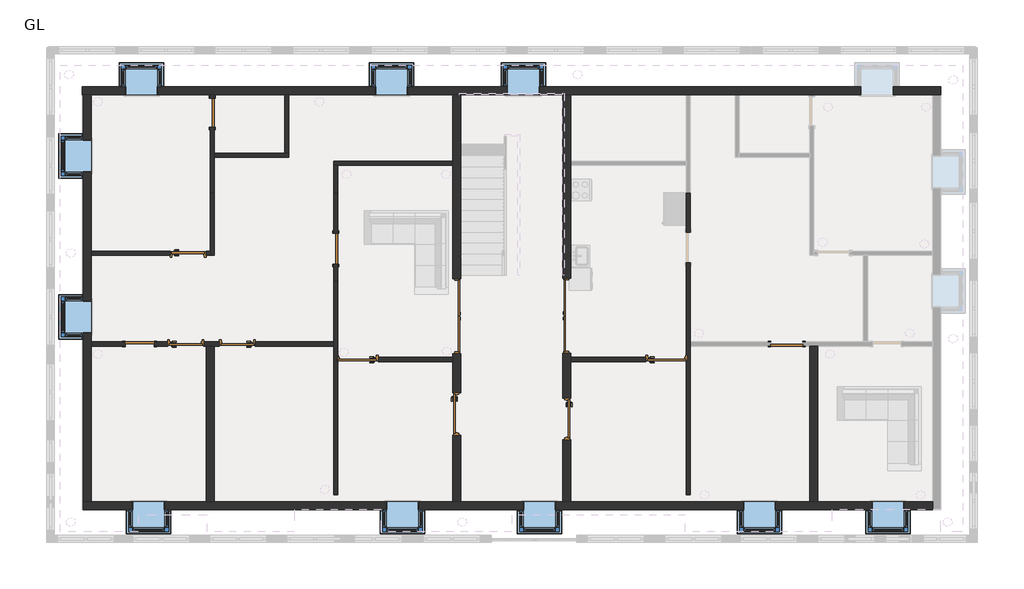
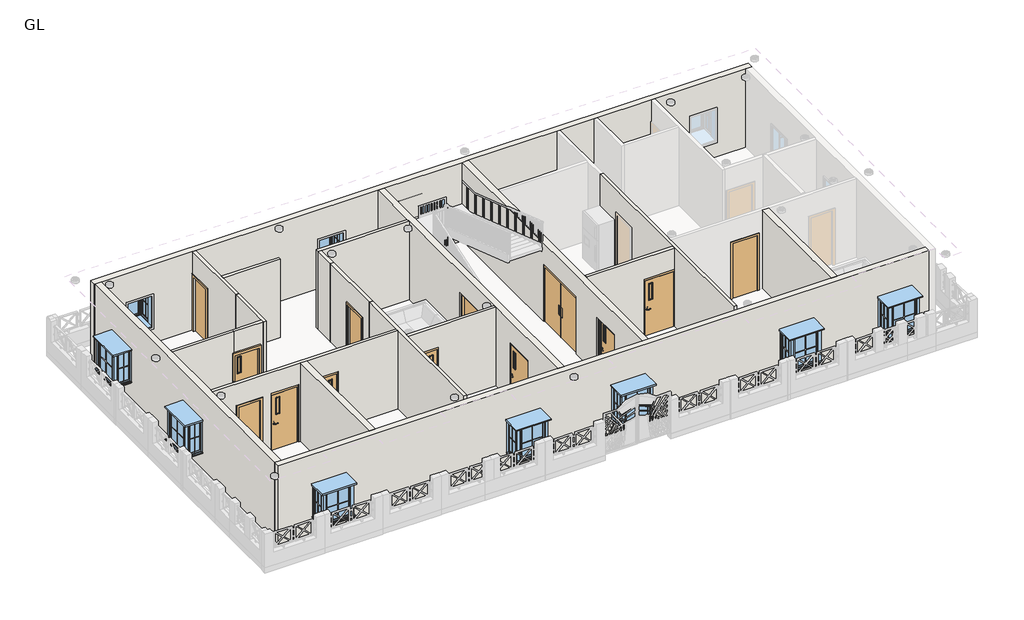
# One storey, part 1 of 5: 21 walls, 13 doors, 10 windows.
"""IFC4 building model written with IfcOpenShell, lengths in millimetres."""

from ifc_helpers import new_model, si_unit, frame, origin, origin_with_axes, place, context, project, spatial, polyline, outline, extrude, faceted_brep, transform, mapped, element, save
from components import door_2c854dd0, door_cf1f2706, door_586e558e, door_4f5842df, door_7d8f8091, door_passage_single_vision_lite_3_x7_440dd290, door_passage_single_vision_lite_3_x7_38248cdf, door_70e57c00, door_8cb1b8a7, door_38851409, door_d141acb4, window_bay_casement_box_90_degree_angle_center_fixed_4_x3_2dea7aab

model = new_model("IFC4")

# Units and contexts
model_context = context("Model", 3, world=origin())
ifc_project = project(units=[si_unit("LENGTHUNIT", "METRE", prefix="MILLI")], contexts=[model_context])

# Site, building, storey
site = spatial("IfcSite", under=ifc_project)
building = spatial("IfcBuilding", under=site)
storey = spatial("IfcBuildingStorey", under=building, Name="GL", Elevation=0.0)

# Doors
placement = place(None, origin())
door_shape = door_2c854dd0(model_context)
element("IfcDoor", 1, ObjectType="Door-Passage-Double-Flush-Dbl_Acting : 6'79\" X 84\"", at=placement, inside=storey, context=model_context, shape_type="MappedRepresentation", body=[
    mapped(door_shape, transform((-1969.4487998, 1424.4578621, 0.0), x_axis=(0.0, -1.0, 0.0), y_axis=(1.0, 0.0, 0.0), z_axis=(0.0, 0.0, 1.0))),
])
element("IfcDoor", 2, ObjectType="Door-Passage-Double-Flush-Dbl_Acting : 6'79\" X 84\"", at=placement, inside=storey, context=model_context, shape_type="MappedRepresentation", body=[
    mapped(door_shape, transform((1128.8432011, 1434.2067807, 0.0), x_axis=(0.0, 1.0, 0.0), y_axis=(-1.0, 0.0, 0.0), z_axis=(0.0, 0.0, 1.0))),
])
door_2_shape = door_cf1f2706(model_context)
element("IfcDoor", 3, ObjectType="Door-Passage-Single-Vision_Lite : 3'6\"X7' 2", at=placement, inside=storey, context=model_context, shape_type="MappedRepresentation", body=[
    mapped(door_2_shape, transform((-4750.7487995, 211.6078621, 0.0), x_axis=(-1.0, 0.0, 0.0), y_axis=(0.0, -1.0, 0.0), z_axis=(0.0, 0.0, 1.0))),
])
door_3_shape = door_586e558e(model_context)
element("IfcDoor", 4, ObjectType="Door-Passage-Single-Vision_Lite : 3'6\"X7' 2", at=placement, inside=storey, context=model_context, shape_type="MappedRepresentation", body=[
    mapped(door_3_shape, transform((1116.1432011, -1461.3932193, 0.0), x_axis=(0.0, -1.0, 0.0), y_axis=(1.0, 0.0, 0.0), z_axis=(0.0, 0.0, 1.0))),
])
door_4_shape = door_4f5842df(model_context)
element("IfcDoor", 5, ObjectType="Door-Passage-Single-Vision_Lite : 3'6\"X7' 2", at=placement, inside=storey, context=model_context, shape_type="MappedRepresentation", body=[
    mapped(door_4_shape, transform((3923.3512082, 211.6078621, 0.0), x_axis=(1.0, 0.0, 0.0), y_axis=(0.0, 1.0, 0.0), z_axis=(0.0, 0.0, 1.0))),
])
door_5_shape = door_7d8f8091(model_context)
element("IfcDoor", 6, ObjectType="Door-Passage-Single-Vision_Lite : 3'7\"X7' 3", at=placement, inside=storey, context=model_context, shape_type="MappedRepresentation", body=[
    mapped(door_5_shape, transform((-1956.7487998, -1318.7421379, 0.0), x_axis=(0.0, -1.0, 0.0), y_axis=(1.0, 0.0, 0.0), z_axis=(0.0, 0.0, 1.0))),
])
door_passage_single_vision_lite_3_x7_shape = door_passage_single_vision_lite_3_x7_440dd290(model_context)
element("IfcDoor", 7, ObjectType="Door-Passage-Single-Vision_Lite : 3'X7'", at=placement, inside=storey, context=model_context, shape_type="MappedRepresentation", body=[
    mapped(door_passage_single_vision_lite_3_x7_shape, transform((-9501.8462614, 3186.8067332, 0.0), x_axis=(1.0, 0.0, 0.0), y_axis=(0.0, 1.0, 0.0), z_axis=(0.0, 0.0, 1.0))),
])
element("IfcDoor", 8, ObjectType="Door-Passage-Single-Vision_Lite : 3'X7'", at=placement, inside=storey, context=model_context, shape_type="MappedRepresentation", body=[
    mapped(door_passage_single_vision_lite_3_x7_shape, transform((-8122.5987992, 646.8067334, 0.0), x_axis=(-1.0, 0.0, 0.0), y_axis=(0.0, -1.0, 0.0), z_axis=(0.0, 0.0, 1.0))),
])
door_passage_single_vision_lite_3_x7_2_shape = door_passage_single_vision_lite_3_x7_38248cdf(model_context)
element("IfcDoor", 9, ObjectType="Door-Passage-Single-Vision_Lite : 3'X7'", at=placement, inside=storey, context=model_context, shape_type="MappedRepresentation", body=[
    mapped(door_passage_single_vision_lite_3_x7_2_shape, transform((-9570.3987992, 646.8067334, 0.0), x_axis=(1.0, 0.0, 0.0), y_axis=(0.0, 1.0, 0.0), z_axis=(0.0, 0.0, 1.0))),
])
door_6_shape = door_70e57c00(model_context)
element("IfcDoor", 10, ObjectType="Single-Flush : 2'10\" x 7'", at=placement, inside=storey, context=model_context, shape_type="MappedRepresentation", body=[
    mapped(door_6_shape, transform((-5360.3487995, 3313.8067802, 0.0), x_axis=(0.0, -1.0, 0.0), y_axis=(1.0, 0.0, 0.0), z_axis=(0.0, 0.0, 1.0))),
])
door_7_shape = door_8cb1b8a7(model_context)
element("IfcDoor", 11, ObjectType="Single-Flush : 2'11\"x 7'", at=placement, inside=storey, context=model_context, shape_type="MappedRepresentation", body=[
    mapped(door_7_shape, transform((7295.2012079, 640.4567334, 0.0), x_axis=(1.0, 0.0, 0.0), y_axis=(0.0, 1.0, 0.0), z_axis=(0.0, 0.0, 1.0))),
])
door_8_shape = door_38851409(model_context)
element("IfcDoor", 12, ObjectType="Single-Flush : 2'8\"x 7'", at=placement, inside=storey, context=model_context, shape_type="MappedRepresentation", body=[
    mapped(door_8_shape, transform((-8827.4487992, 7136.5067329, 0.0), x_axis=(0.0, 1.0, 0.0), y_axis=(-1.0, 0.0, 0.0), z_axis=(0.0, 0.0, 1.0))),
])
door_9_shape = door_d141acb4(model_context)
element("IfcDoor", 13, ObjectType="Single-Flush : 2'8\"x 7'", at=placement, inside=storey, context=model_context, shape_type="MappedRepresentation", body=[
    mapped(door_9_shape, transform((-10865.7987992, 640.4567334, 0.0), x_axis=(1.0, 0.0, 0.0), y_axis=(0.0, 1.0, 0.0), z_axis=(0.0, 0.0, 1.0))),
])

# Walls
element("IfcWall", 14, ObjectType="Generic - 4.5\"", at=placement, inside=storey, context=model_context, shape_type="SweptSolid", body=[
    extrude(outline(polyline([(3048.0, -9959.0462614), (3048.0, -12224.6987925), (0.0, -12224.6987925), (0.0, -10009.8462614), (2235.2, -10009.8462614), (2235.2, -9959.0462614), (3048.0, -9959.0462614)])), frame((0.0, 3136.0067332, 0.0), z_axis=(0.0, 1.0, 0.0), x_axis=(0.0, 0.0, 1.0)), (0.0, 0.0, 1.0), 114.3),
])
element("IfcWall", 15, ObjectType="Generic - 4.5\"", at=placement, inside=storey, context=model_context, shape_type="Brep", body=[
    faceted_brep([(-8884.5987992, 4875.906733, 0.0), (-8884.5987992, 3250.3067332, 0.0), (-8884.5987992, 3136.0067332, 0.0), (-8884.5987992, 3136.0067332, 3048.0), (-8884.5987992, 3250.3067332, 3048.0), (-8884.5987992, 4875.906733, 3048.0), (-8770.2987992, 4875.906733, 0.0), (-8770.2987992, 4875.906733, 3048.0), (-8770.2987992, 3136.0067332, 3048.0), (-8770.2987992, 3136.0067332, 0.0)], [[[0, 1, 2, 3, 4, 5]], [[6, 7, 8, 9]], [[2, 1, 0, 6, 9]], [[5, 4, 3, 8, 7]], [[0, 5, 7, 6]], [[3, 2, 9, 8]]]),
])
element("IfcWall", 16, ObjectType="Generic - 4.5\"", at=placement, inside=storey, context=model_context, shape_type="Brep", body=[
    faceted_brep([(-10459.3987992, 583.3067334, 2133.6), (-10459.3987992, 583.3067334, 0.0), (-10078.3987992, 583.3067334, 0.0), (-10078.3987992, 583.3067334, 2235.2), (-9062.3987992, 583.3067334, 2235.2), (-9062.3987992, 583.3067334, 0.0), (-8998.8987992, 583.3067334, 0.0), (-8770.2987992, 583.3067334, 0.0), (-8630.5987992, 583.3067334, 0.0), (-8630.5987992, 583.3067334, 2235.2), (-7614.5987992, 583.3067334, 2235.2), (-7614.5987992, 583.3067334, 0.0), (-5417.4987995, 583.3067334, 0.0), (-5417.4987995, 583.3067334, 3048.0), (-8770.2987992, 583.3067334, 3048.0), (-8998.8987992, 583.3067334, 3048.0), (-12224.6987925, 583.3067334, 3048.0), (-12224.6987925, 583.3067334, 0.0), (-11272.1987992, 583.3067334, 0.0), (-11272.1987992, 583.3067334, 2133.6), (-10078.3987992, 697.6067334, 0.0), (-10459.3987992, 697.6067334, 0.0), (-10459.3987992, 697.6067334, 2133.6), (-11272.1987992, 697.6067334, 2133.6), (-11272.1987992, 697.6067334, 0.0), (-12224.6987925, 697.6067334, 0.0), (-12224.6987925, 697.6067334, 3048.0), (-5417.4987995, 697.6067334, 3048.0), (-5417.4987995, 697.6067334, 0.0), (-7614.5987992, 697.6067334, 0.0), (-7614.5987992, 697.6067334, 2235.2), (-8630.5987992, 697.6067334, 2235.2), (-8630.5987992, 697.6067334, 0.0), (-9062.3987992, 697.6067334, 0.0), (-9062.3987992, 697.6067334, 2235.2), (-10078.3987992, 697.6067334, 2235.2)], [[[0, 1, 2, 3, 4, 5, 6, 7, 8, 9, 10, 11, 12, 13, 14, 15, 16, 17, 18, 19]], [[20, 21, 22, 23, 24, 25, 26, 27, 28, 29, 30, 31, 32, 33, 34, 35]], [[28, 12, 11, 29]], [[32, 8, 7, 6, 5, 33]], [[18, 17, 25, 24]], [[2, 1, 21, 20]], [[16, 15, 14, 13, 27, 26]], [[17, 16, 26, 25]], [[13, 12, 28, 27]], [[9, 8, 32, 31]], [[10, 9, 31, 30]], [[11, 10, 30, 29]], [[4, 34, 33, 5]], [[34, 4, 3, 35]], [[35, 3, 2, 20]], [[22, 21, 1, 0]], [[23, 22, 0, 19]], [[24, 23, 19, 18]]]),
])
element("IfcWall", 17, ObjectType="Generic - 4.5\"", at=placement, inside=storey, context=model_context, shape_type="SweptSolid", body=[
    extrude(outline(polyline([(3048.0, -2077.3987998), (3048.0, -5303.1987995), (2235.2, -5303.1987995), (2235.2, -4166.5487995), (0.0, -4166.5487995), (0.0, -2077.3987998), (3048.0, -2077.3987998)])), frame((0.0, 148.1078621, 0.0), z_axis=(0.0, 1.0, 0.0), x_axis=(0.0, 0.0, 1.0)), (0.0, 0.0, 1.0), 114.3),
])
element("IfcWall", 18, ObjectType="Generic - 4.5\"", at=placement, inside=storey, context=model_context, shape_type="Brep", body=[
    faceted_brep([(-5417.4987995, 2399.4067802, 0.0), (-5417.4987995, 697.6067334, 0.0), (-5417.4987995, 583.3067334, 0.0), (-5417.4987995, -3594.9932193, 0.0), (-5417.4987995, -3594.9932193, 3048.0), (-5417.4987995, 583.3067334, 3048.0), (-5417.4987995, 697.6067334, 3048.0), (-5417.4987995, 2399.4067802, 3048.0), (-5303.1987995, -3594.9932193, 3048.0), (-5303.1987995, -3594.9932193, 0.0), (-5303.1987995, 148.1078621, 0.0), (-5303.1987995, 148.1078621, 2235.2), (-5303.1987995, 262.4078621, 2235.2), (-5303.1987995, 262.4078621, 0.0), (-5303.1987995, 2399.4067802, 0.0), (-5303.1987995, 2399.4067802, 3048.0), (-5303.1987995, 262.4078621, 3048.0), (-5303.1987995, 148.1078621, 3048.0), (-5334.9487995, 262.4078621, 0.0), (-5334.9487995, 148.1078621, 0.0), (-5334.9487995, 262.4078621, 2235.2), (-5334.9487995, 148.1078621, 2235.2)], [[[0, 1, 2, 3, 4, 5, 6, 7]], [[8, 9, 10, 11, 12, 13, 14, 15, 16, 17]], [[3, 2, 1, 0, 14, 13, 18, 19, 10, 9]], [[4, 3, 9, 8]], [[7, 6, 5, 4, 8, 17, 16, 15]], [[0, 7, 15, 14]], [[20, 18, 13, 12]], [[19, 21, 11, 10]], [[21, 20, 12, 11]], [[18, 20, 21, 19]]]),
])
element("IfcWall", 19, ObjectType="Generic - 4.5\"", at=placement, inside=storey, context=model_context, shape_type="Brep", body=[
    faceted_brep([(-2077.3987998, 5764.9067329, 0.0), (-5417.4987995, 5764.9067329, 0.0), (-5417.4987995, 5764.9067329, 3048.0), (-2077.3987998, 5764.9067329, 3048.0), (-2077.3987998, 5650.6067329, 0.0), (-2077.3987998, 5650.6067329, 3048.0), (-5303.1987995, 5650.6067329, 3048.0), (-5417.4987995, 5650.6067329, 3048.0), (-5417.4987995, 5650.6067329, 0.0), (-5303.1987995, 5650.6067329, 0.0)], [[[0, 1, 2, 3]], [[4, 5, 6, 7, 8, 9]], [[1, 0, 4, 9, 8]], [[3, 2, 7, 6, 5]], [[2, 1, 8, 7]], [[0, 3, 5, 4]]]),
])
element("IfcWall", 20, ObjectType="Generic - 4.5\"", at=placement, inside=storey, context=model_context, shape_type="SweptSolid", body=[
    extrude(outline(polyline([(-5417.4987995, 4875.90678), (-5417.4987995, 5650.6067329), (-5303.1987995, 5650.6067329), (-5303.1987995, 4875.90678), (-5417.4987995, 4875.90678)])), origin_with_axes(), (0.0, 0.0, 1.0), 3048.0),
])
element("IfcWall", 21, ObjectType="Generic - 4.5\"", at=placement, inside=storey, context=model_context, shape_type="Brep", body=[
    faceted_brep([(4475.8012082, -3594.9932193, 0.0), (4475.8012082, -3594.9932193, 3048.0), (4475.8012082, 148.1078621, 3048.0), (4475.8012082, 262.4078621, 3048.0), (4475.8012082, 4875.906733, 3048.0), (4475.8012082, 4875.906733, 0.0), (4475.8012082, 3783.706733, 0.0), (4475.8012082, 3783.706733, 2133.6), (4475.8012082, 2920.106733, 2133.6), (4475.8012082, 2920.106733, 0.0), (4475.8012082, 262.4078621, 0.0), (4475.8012082, 262.4078621, 2235.2), (4475.8012082, 148.1078621, 2235.2), (4475.8012082, 148.1078621, 0.0), (4590.1012082, -3594.9932193, 3048.0), (4590.1012082, -3594.9932193, 0.0), (4590.1012082, 583.3067334, 0.0), (4590.1012082, 697.6067334, 0.0), (4590.1012082, 2920.106733, 0.0), (4590.1012082, 2920.106733, 2133.6), (4590.1012082, 3783.706733, 2133.6), (4590.1012082, 3783.706733, 0.0), (4590.1012082, 4875.906733, 0.0), (4590.1012082, 4875.906733, 3048.0), (4590.1012082, 697.6067334, 3048.0), (4590.1012082, 583.3067334, 3048.0), (4507.5512082, 148.1078621, 0.0), (4507.5512082, 262.4078621, 0.0), (4507.5512082, 148.1078621, 2235.2), (4507.5512082, 262.4078621, 2235.2)], [[[0, 1, 2, 3, 4, 5, 6, 7, 8, 9, 10, 11, 12, 13]], [[14, 15, 16, 17, 18, 19, 20, 21, 22, 23, 24, 25]], [[15, 0, 13, 26, 27, 10, 9, 18, 17, 16]], [[5, 22, 21, 6]], [[1, 0, 15, 14]], [[4, 3, 2, 1, 14, 25, 24, 23]], [[5, 4, 23, 22]], [[19, 18, 9, 8]], [[20, 19, 8, 7]], [[21, 20, 7, 6]], [[28, 26, 13, 12]], [[27, 29, 11, 10]], [[26, 28, 29, 27]], [[29, 28, 12, 11]]]),
])
element("IfcWall", 22, ObjectType="Generic - 4.5\"", at=placement, inside=storey, context=model_context, shape_type="Brep", body=[
    faceted_brep([(-8770.2987992, 7542.9067329, 2133.6), (-8770.2987992, 7542.9067329, 0.0), (-8770.2987992, 7631.8067329, 0.0), (-8770.2987992, 7631.8067329, 3048.0), (-8770.2987992, 5993.5067329, 3048.0), (-8770.2987992, 5879.2067329, 3048.0), (-8770.2987992, 4875.906733, 3048.0), (-8770.2987992, 4875.906733, 0.0), (-8770.2987992, 5879.2067329, 0.0), (-8770.2987992, 5993.5067329, 0.0), (-8770.2987992, 6730.1067329, 0.0), (-8770.2987992, 6730.1067329, 2133.6), (-8884.5987992, 7631.8067329, 0.0), (-8884.5987992, 7542.9067329, 0.0), (-8884.5987992, 7542.9067329, 2133.6), (-8884.5987992, 6730.1067329, 2133.6), (-8884.5987992, 6730.1067329, 0.0), (-8884.5987992, 4875.906733, 0.0), (-8884.5987992, 4875.906733, 3048.0), (-8884.5987992, 7631.8067329, 3048.0)], [[[0, 1, 2, 3, 4, 5, 6, 7, 8, 9, 10, 11]], [[12, 13, 14, 15, 16, 17, 18, 19]], [[2, 1, 13, 12]], [[10, 9, 8, 7, 17, 16]], [[6, 5, 4, 3, 19, 18]], [[7, 6, 18, 17]], [[3, 2, 12, 19]], [[14, 13, 1, 0]], [[15, 14, 0, 11]], [[16, 15, 11, 10]]]),
])
element("IfcWall", 23, ObjectType="Generic - 4.5\"", at=placement, inside=storey, context=model_context, shape_type="Brep", body=[
    faceted_brep([(-8770.2987992, 5879.2067329, 0.0), (-6674.7987994, 5879.2067329, 0.0), (-6674.7987994, 5879.2067329, 3048.0), (-8770.2987992, 5879.2067329, 3048.0), (-8770.2987992, 5993.5067329, 0.0), (-8770.2987992, 5993.5067329, 3048.0), (-6674.7987994, 5993.5067329, 3048.0), (-6674.7987994, 5993.5067329, 1371.6), (-6674.7987994, 5993.5067329, 0.0), (-6789.0987994, 5993.5067329, 0.0)], [[[0, 1, 2, 3]], [[4, 5, 6, 7, 8, 9]], [[1, 0, 4, 9, 8]], [[3, 2, 6, 5]], [[0, 3, 5, 4]], [[2, 1, 8, 7, 6]]]),
])
element("IfcWall", 24, ObjectType="Generic - 4.5\"", at=placement, inside=storey, context=model_context, shape_type="SweptSolid", body=[
    extrude(outline(polyline([(-6674.7987994, 7631.8067329), (-6674.7987994, 5993.5067329), (-6789.0987994, 5993.5067329), (-6789.0987994, 7631.8067329), (-6674.7987994, 7631.8067329)])), origin_with_axes(), (0.0, 0.0, 1.0), 1371.6),
])
element("IfcWall", 25, ObjectType="Generic - 4.5\"", at=placement, inside=storey, context=model_context, shape_type="SweptSolid", body=[
    extrude(outline(polyline([(3048.0, -8884.5987992), (3048.0, -9959.0462614), (2235.2, -9959.0462614), (2235.2, -8993.8462614), (0.0, -8993.8462614), (0.0, -8884.5987992), (3048.0, -8884.5987992)])), frame((0.0, 3136.0067332, 0.0), z_axis=(0.0, 1.0, 0.0), x_axis=(0.0, 0.0, 1.0)), (0.0, 0.0, 1.0), 114.3),
])
element("IfcWall", 26, ObjectType="Generic - 4.5\"", at=placement, inside=storey, context=model_context, shape_type="SweptSolid", body=[
    extrude(outline(polyline([(2882.0067802, 2133.6), (2882.0067802, 0.0), (2399.4067802, 0.0), (2399.4067802, 3048.0), (4875.90678, 3048.0), (4875.90678, 0.0), (3745.6067802, 0.0), (3745.6067802, 2133.6), (2882.0067802, 2133.6)])), frame((-5417.4987995, 0.0, 0.0), z_axis=(1.0, 0.0, 0.0), x_axis=(0.0, 1.0, 0.0)), (0.0, 0.0, 1.0), 114.3),
])
element("IfcWall", 27, ObjectType="Generic - 4.5\"", at=placement, inside=storey, context=model_context, shape_type="SweptSolid", body=[
    extrude(outline(polyline([(3048.0, 4475.8012082), (3048.0, 1250.0012085), (0.0, 1250.0012085), (0.0, 3339.1512082), (2235.2, 3339.1512082), (2235.2, 4475.8012082), (3048.0, 4475.8012082)])), frame((0.0, 148.1078621, 0.0), z_axis=(0.0, 1.0, 0.0), x_axis=(0.0, 0.0, 1.0)), (0.0, 0.0, 1.0), 114.3),
])
element("IfcWall", 28, ObjectType="Generic - 9\"", at=placement, inside=storey, context=model_context, shape_type="Brep", body=[
    faceted_brep([(-12479.2067989, 7631.8067329, 0.0), (-12453.2987925, 7631.8067329, 0.0), (-12224.6987925, 7631.8067329, 0.0), (-8884.5987992, 7631.8067329, 0.0), (-8770.2987992, 7631.8067329, 0.0), (-6789.0987994, 7631.8067329, 0.0), (-6674.7987994, 7631.8067329, 0.0), (-2077.3987998, 7631.8067329, 0.0), (-1848.7987998, 7631.8067329, 0.0), (1008.1932011, 7631.8067329, 0.0), (1236.7932011, 7631.8067329, 0.0), (4475.8012082, 7631.8067329, 0.0), (4590.1012082, 7631.8067329, 0.0), (5847.401208, 7631.8067329, 0.0), (5961.701208, 7631.8067329, 0.0), (11397.3012075, 7631.8067329, 0.0), (11625.9012075, 7631.8067329, 0.0), (11625.9012075, 7631.8067329, 3048.0), (11397.3012075, 7631.8067329, 3048.0), (5961.701208, 7631.8067329, 3048.0), (5847.401208, 7631.8067329, 3048.0), (4590.1012082, 7631.8067329, 3048.0), (4475.8012082, 7631.8067329, 3048.0), (1236.7932011, 7631.8067329, 3048.0), (1008.1932011, 7631.8067329, 3048.0), (-1848.7987998, 7631.8067329, 3048.0), (-2077.3987998, 7631.8067329, 3048.0), (-8770.2987992, 7631.8067329, 3048.0), (-8884.5987992, 7631.8067329, 3048.0), (-12224.6987925, 7631.8067329, 3048.0), (-12453.2987925, 7631.8067329, 3048.0), (-12479.2067989, 7631.8067329, 3048.0), (-10357.7987925, 7631.8067329, 1879.6), (-10357.7987925, 7631.8067329, 609.6), (-11272.1987925, 7631.8067329, 609.6), (-11272.1987925, 7631.8067329, 1879.6), (-3334.6987998, 7631.8067329, 1879.6), (-3334.6987998, 7631.8067329, 609.6), (-4249.0987998, 7631.8067329, 609.6), (-4249.0987998, 7631.8067329, 1879.6), (360.4932011, 7631.8067329, 1879.6), (360.4932011, 7631.8067329, 609.6), (-553.9067989, 7631.8067329, 609.6), (-553.9067989, 7631.8067329, 1879.6), (10292.4012075, 7631.8067329, 1879.6), (10292.4012075, 7631.8067329, 609.6), (9378.0012075, 7631.8067329, 609.6), (9378.0012075, 7631.8067329, 1879.6), (-12479.2067989, 7860.4067329, 0.0), (-12479.2067989, 7860.4067329, 3048.0), (11625.9012075, 7860.4067329, 3048.0), (11625.9012075, 7860.4067329, 0.0), (-10357.7987925, 7860.4067329, 1879.6), (-11272.1987925, 7860.4067329, 1879.6), (-11272.1987925, 7860.4067329, 609.6), (-10357.7987925, 7860.4067329, 609.6), (-3334.6987998, 7860.4067329, 1879.6), (-4249.0987998, 7860.4067329, 1879.6), (-4249.0987998, 7860.4067329, 609.6), (-3334.6987998, 7860.4067329, 609.6), (360.4932011, 7860.4067329, 1879.6), (-553.9067989, 7860.4067329, 1879.6), (-553.9067989, 7860.4067329, 609.6), (360.4932011, 7860.4067329, 609.6), (10292.4012075, 7860.4067329, 1879.6), (9378.0012075, 7860.4067329, 1879.6), (9378.0012075, 7860.4067329, 609.6), (10292.4012075, 7860.4067329, 609.6)], [[[0, 1, 2, 3, 4, 5, 6, 7, 8, 9, 10, 11, 12, 13, 14, 15, 16, 17, 18, 19, 20, 21, 22, 23, 24, 25, 26, 27, 28, 29, 30, 31], [32, 33, 34, 35], [36, 37, 38, 39], [40, 41, 42, 43], [44, 45, 46, 47]], [[48, 49, 50, 51], [52, 53, 54, 55], [56, 57, 58, 59], [60, 61, 62, 63], [64, 65, 66, 67]], [[16, 15, 14, 13, 12, 11, 10, 9, 8, 7, 6, 5, 4, 3, 2, 1, 0, 48, 51]], [[31, 30, 29, 28, 27, 26, 25, 24, 23, 22, 21, 20, 19, 18, 17, 50, 49]], [[0, 31, 49, 48]], [[17, 16, 51, 50]], [[33, 32, 52, 55]], [[34, 33, 55, 54]], [[35, 34, 54, 53]], [[32, 35, 53, 52]], [[37, 36, 56, 59]], [[38, 37, 59, 58]], [[39, 38, 58, 57]], [[36, 39, 57, 56]], [[41, 40, 60, 63]], [[42, 41, 63, 62]], [[43, 42, 62, 61]], [[40, 43, 61, 60]], [[45, 44, 64, 67]], [[46, 45, 67, 66]], [[47, 46, 66, 65]], [[44, 47, 65, 64]]]),
])
element("IfcWall", 29, ObjectType="Generic - 9\"", at=placement, inside=storey, context=model_context, shape_type="Brep", body=[
    faceted_brep([(11397.3012075, -3785.4932193, 0.0), (8171.5012079, -3785.4932193, 0.0), (7942.9012079, -3785.4932193, 0.0), (1236.7932011, -3785.4932193, 0.0), (1008.1932011, -3785.4932193, 0.0), (-1848.7987998, -3785.4932193, 0.0), (-2077.3987998, -3785.4932193, 0.0), (-8770.2987992, -3785.4932193, 0.0), (-8998.8987992, -3785.4932193, 0.0), (-12224.6987925, -3785.4932193, 0.0), (-12453.2987925, -3785.4932193, 0.0), (-12453.2987925, -3785.4932193, 3048.0), (-12224.6987925, -3785.4932193, 3048.0), (-8998.8987992, -3785.4932193, 3048.0), (-8770.2987992, -3785.4932193, 3048.0), (-2077.3987998, -3785.4932193, 3048.0), (-1848.7987998, -3785.4932193, 3048.0), (1008.1932011, -3785.4932193, 3048.0), (1236.7932011, -3785.4932193, 3048.0), (7942.9012079, -3785.4932193, 3048.0), (8171.5012079, -3785.4932193, 3048.0), (11397.3012075, -3785.4932193, 3048.0), (-11068.9987958, -3785.4932193, 1879.6), (-11068.9987958, -3785.4932193, 609.6), (-10154.5987958, -3785.4932193, 609.6), (-10154.5987958, -3785.4932193, 1879.6), (-3944.2987998, -3785.4932193, 1879.6), (-3944.2987998, -3785.4932193, 609.6), (-3029.8987998, -3785.4932193, 609.6), (-3029.8987998, -3785.4932193, 1879.6), (-96.7067989, -3785.4932193, 1879.6), (-96.7067989, -3785.4932193, 609.6), (817.6932011, -3785.4932193, 609.6), (817.6932011, -3785.4932193, 1879.6), (6076.0012079, -3785.4932193, 1879.6), (6076.0012079, -3785.4932193, 609.6), (6990.4012079, -3785.4932193, 609.6), (6990.4012079, -3785.4932193, 1879.6), (9682.8012075, -3785.4932193, 1879.6), (9682.8012075, -3785.4932193, 609.6), (10597.2012075, -3785.4932193, 609.6), (10597.2012075, -3785.4932193, 1879.6), (11397.3012075, -4014.0932193, 0.0), (11397.3012075, -4014.0932193, 3048.0), (-12453.2987925, -4014.0932193, 3048.0), (-12453.2987925, -4014.0932193, 0.0), (-11068.9987958, -4014.0932193, 1879.6), (-10154.5987958, -4014.0932193, 1879.6), (-10154.5987958, -4014.0932193, 609.6), (-11068.9987958, -4014.0932193, 609.6), (-3944.2987998, -4014.0932193, 1879.6), (-3029.8987998, -4014.0932193, 1879.6), (-3029.8987998, -4014.0932193, 609.6), (-3944.2987998, -4014.0932193, 609.6), (-96.7067989, -4014.0932193, 1879.6), (817.6932011, -4014.0932193, 1879.6), (817.6932011, -4014.0932193, 609.6), (-96.7067989, -4014.0932193, 609.6), (6076.0012079, -4014.0932193, 1879.6), (6990.4012079, -4014.0932193, 1879.6), (6990.4012079, -4014.0932193, 609.6), (6076.0012079, -4014.0932193, 609.6), (9682.8012075, -4014.0932193, 1879.6), (10597.2012075, -4014.0932193, 1879.6), (10597.2012075, -4014.0932193, 609.6), (9682.8012075, -4014.0932193, 609.6)], [[[0, 1, 2, 3, 4, 5, 6, 7, 8, 9, 10, 11, 12, 13, 14, 15, 16, 17, 18, 19, 20, 21], [22, 23, 24, 25], [26, 27, 28, 29], [30, 31, 32, 33], [34, 35, 36, 37], [38, 39, 40, 41]], [[42, 43, 44, 45], [46, 47, 48, 49], [50, 51, 52, 53], [54, 55, 56, 57], [58, 59, 60, 61], [62, 63, 64, 65]], [[10, 9, 8, 7, 6, 5, 4, 3, 2, 1, 0, 42, 45]], [[21, 20, 19, 18, 17, 16, 15, 14, 13, 12, 11, 44, 43]], [[0, 21, 43, 42]], [[11, 10, 45, 44]], [[23, 22, 46, 49]], [[24, 23, 49, 48]], [[25, 24, 48, 47]], [[22, 25, 47, 46]], [[27, 26, 50, 53]], [[28, 27, 53, 52]], [[29, 28, 52, 51]], [[26, 29, 51, 50]], [[31, 30, 54, 57]], [[32, 31, 57, 56]], [[33, 32, 56, 55]], [[30, 33, 55, 54]], [[35, 34, 58, 61]], [[36, 35, 61, 60]], [[37, 36, 60, 59]], [[34, 37, 59, 58]], [[39, 38, 62, 65]], [[40, 39, 65, 64]], [[41, 40, 64, 63]], [[38, 41, 63, 62]]]),
])
element("IfcWall", 30, ObjectType="Generic - 9\"", at=placement, inside=storey, context=model_context, shape_type="Brep", body=[
    faceted_brep([(-12224.6987925, -3785.4932193, 0.0), (-12224.6987925, 583.3067334, 0.0), (-12224.6987925, 697.6067334, 0.0), (-12224.6987925, 3136.0067332, 0.0), (-12224.6987925, 3250.3067332, 0.0), (-12224.6987925, 7631.8067329, 0.0), (-12224.6987925, 7631.8067329, 3048.0), (-12224.6987925, 3250.3067332, 3048.0), (-12224.6987925, 3136.0067332, 3048.0), (-12224.6987925, 697.6067334, 3048.0), (-12224.6987925, 583.3067334, 3048.0), (-12224.6987925, -3785.4932193, 3048.0), (-12224.6987925, 1859.6567334, 1879.6), (-12224.6987925, 1859.6567334, 609.6), (-12224.6987925, 945.2567334, 609.6), (-12224.6987925, 945.2567334, 1879.6), (-12224.6987925, 6374.5067329, 1879.6), (-12224.6987925, 6374.5067329, 609.6), (-12224.6987925, 5460.1067329, 609.6), (-12224.6987925, 5460.1067329, 1879.6), (-12453.2987925, -3785.4932193, 0.0), (-12453.2987925, -3785.4932193, 3048.0), (-12453.2987925, 7631.8067329, 3048.0), (-12453.2987925, 7631.8067329, 0.0), (-12453.2987925, 1859.6567334, 1879.6), (-12453.2987925, 945.2567334, 1879.6), (-12453.2987925, 945.2567334, 609.6), (-12453.2987925, 1859.6567334, 609.6), (-12453.2987925, 6374.5067329, 1879.6), (-12453.2987925, 5460.1067329, 1879.6), (-12453.2987925, 5460.1067329, 609.6), (-12453.2987925, 6374.5067329, 609.6)], [[[0, 1, 2, 3, 4, 5, 6, 7, 8, 9, 10, 11], [12, 13, 14, 15], [16, 17, 18, 19]], [[20, 21, 22, 23], [24, 25, 26, 27], [28, 29, 30, 31]], [[5, 4, 3, 2, 1, 0, 20, 23]], [[11, 10, 9, 8, 7, 6, 22, 21]], [[0, 11, 21, 20]], [[6, 5, 23, 22]], [[13, 12, 24, 27]], [[14, 13, 27, 26]], [[15, 14, 26, 25]], [[12, 15, 25, 24]], [[17, 16, 28, 31]], [[18, 17, 31, 30]], [[19, 18, 30, 29]], [[16, 19, 29, 28]]]),
])
element("IfcWall", 31, ObjectType="Generic - 9\"", at=placement, inside=storey, context=model_context, shape_type="SweptSolid", body=[
    extrude(outline(polyline([(-8998.8987992, -3785.4932193), (-8998.8987992, 583.3067334), (-8770.2987992, 583.3067334), (-8770.2987992, -3785.4932193), (-8998.8987992, -3785.4932193)])), origin_with_axes(), (0.0, 0.0, 1.0), 3048.0),
])
element("IfcWall", 32, ObjectType="Generic - 9\"", at=placement, inside=storey, context=model_context, shape_type="Brep", body=[
    faceted_brep([(-2077.3987998, -3785.4932193, 3048.0), (-2077.3987998, 148.1078621, 3048.0), (-2077.3987998, 262.4078621, 3048.0), (-2077.3987998, 5650.6067329, 3048.0), (-2077.3987998, 5764.9067329, 3048.0), (-2077.3987998, 7631.8067329, 3048.0), (-2077.3987998, 7631.8067329, 0.0), (-2077.3987998, 5764.9067329, 0.0), (-2077.3987998, 5650.6067329, 0.0), (-2077.3987998, 2478.5578621, 0.0), (-2077.3987998, 2478.5578621, 2235.2), (-2077.3987998, 370.3578621, 2235.2), (-2077.3987998, 370.3578621, 0.0), (-2077.3987998, 262.4078621, 0.0), (-2077.3987998, 148.1078621, 0.0), (-2077.3987998, -721.8421379, 0.0), (-2077.3987998, -721.8421379, 2235.2), (-2077.3987998, -1915.6421379, 2235.2), (-2077.3987998, -1915.6421379, 0.0), (-2077.3987998, -3785.4932193, 0.0), (-1848.7987998, 7631.8067329, 3048.0), (-1848.7987998, -3785.4932193, 3048.0), (-1848.7987998, -3785.4932193, 0.0), (-1848.7987998, -1915.6421379, 0.0), (-1848.7987998, -1915.6421379, 2235.2), (-1848.7987998, -721.8421379, 2235.2), (-1848.7987998, -721.8421379, 0.0), (-1848.7987998, 370.3578621, 0.0), (-1848.7987998, 370.3578621, 2235.2), (-1848.7987998, 2478.5578621, 2235.2), (-1848.7987998, 2478.5578621, 0.0), (-1848.7987998, 7631.8067329, 0.0)], [[[0, 1, 2, 3, 4, 5, 6, 7, 8, 9, 10, 11, 12, 13, 14, 15, 16, 17, 18, 19]], [[20, 21, 22, 23, 24, 25, 26, 27, 28, 29, 30, 31]], [[22, 19, 18, 23]], [[6, 31, 30, 9, 8, 7]], [[26, 15, 14, 13, 12, 27]], [[5, 4, 3, 2, 1, 0, 21, 20]], [[0, 19, 22, 21]], [[6, 5, 20, 31]], [[17, 24, 23, 18]], [[24, 17, 16, 25]], [[25, 16, 15, 26]], [[11, 28, 27, 12]], [[28, 11, 10, 29]], [[29, 10, 9, 30]]]),
])
element("IfcWall", 33, ObjectType="Generic - 9\"", at=placement, inside=storey, context=model_context, shape_type="SweptSolid", body=[
    extrude(outline(polyline([(-3785.4932193, 3048.0), (7631.8067329, 3048.0), (7631.8067329, 0.0), (2488.3067807, 0.0), (2488.3067807, 2235.2), (380.1067807, 2235.2), (380.1067807, 0.0), (-877.1932193, 0.0), (-877.1932193, 2235.2), (-2045.5932193, 2235.2), (-2045.5932193, 0.0), (-3785.4932193, 0.0), (-3785.4932193, 3048.0)])), frame((1008.1932011, 0.0, 0.0), z_axis=(1.0, 0.0, 0.0), x_axis=(0.0, 1.0, 0.0)), (0.0, 0.0, 1.0), 228.6),
])
element("IfcWall", 34, ObjectType="Generic - 9\"", at=placement, inside=storey, context=model_context, shape_type="SweptSolid", body=[
    extrude(outline(polyline([(7942.9012079, -3785.4932193), (7942.9012079, 583.3067334), (8171.5012079, 583.3067334), (8171.5012079, -3785.4932193), (7942.9012079, -3785.4932193)])), origin_with_axes(), (0.0, 0.0, 1.0), 3048.0),
])

# Windows
window_bay_casement_box_90_degree_angle_center_fixed_4_x3_shape = window_bay_casement_box_90_degree_angle_center_fixed_4_x3_2dea7aab(model_context)
element("IfcWindow", 35, ObjectType="Window-Bay-Casement-Box-90_Degree_Angle-Center_Fixed : 4'X3'", at=placement, inside=storey, context=model_context, shape_type="MappedRepresentation", body=[
    mapped(window_bay_casement_box_90_degree_angle_center_fixed_4_x3_shape, transform((-10814.9987925, 7746.1067329, 0.0), x_axis=(1.0, 0.0, 0.0), y_axis=(0.0, 1.0, 0.0), z_axis=(0.0, 0.0, 1.0))),
])
element("IfcWindow", 36, ObjectType="Window-Bay-Casement-Box-90_Degree_Angle-Center_Fixed : 4'X3'", at=placement, inside=storey, context=model_context, shape_type="MappedRepresentation", body=[
    mapped(window_bay_casement_box_90_degree_angle_center_fixed_4_x3_shape, transform((-3791.8987998, 7746.1067329, 0.0), x_axis=(1.0, 0.0, 0.0), y_axis=(0.0, 1.0, 0.0), z_axis=(0.0, 0.0, 1.0))),
])
element("IfcWindow", 37, ObjectType="Window-Bay-Casement-Box-90_Degree_Angle-Center_Fixed : 4'X3'", at=placement, inside=storey, context=model_context, shape_type="MappedRepresentation", body=[
    mapped(window_bay_casement_box_90_degree_angle_center_fixed_4_x3_shape, transform((-96.7067989, 7746.1067329, 0.0), x_axis=(1.0, 0.0, 0.0), y_axis=(0.0, 1.0, 0.0), z_axis=(0.0, 0.0, 1.0))),
])
element("IfcWindow", 38, ObjectType="Window-Bay-Casement-Box-90_Degree_Angle-Center_Fixed : 4'X3'", at=placement, inside=storey, context=model_context, shape_type="MappedRepresentation", body=[
    mapped(window_bay_casement_box_90_degree_angle_center_fixed_4_x3_shape, transform((-10611.7987958, -3899.7932193, 0.0), x_axis=(-1.0, 0.0, 0.0), y_axis=(0.0, -1.0, 0.0), z_axis=(0.0, 0.0, 1.0))),
])
element("IfcWindow", 39, ObjectType="Window-Bay-Casement-Box-90_Degree_Angle-Center_Fixed : 4'X3'", at=placement, inside=storey, context=model_context, shape_type="MappedRepresentation", body=[
    mapped(window_bay_casement_box_90_degree_angle_center_fixed_4_x3_shape, transform((-3487.0987998, -3899.7932193, 0.0), x_axis=(-1.0, 0.0, 0.0), y_axis=(0.0, -1.0, 0.0), z_axis=(0.0, 0.0, 1.0))),
])
element("IfcWindow", 40, ObjectType="Window-Bay-Casement-Box-90_Degree_Angle-Center_Fixed : 4'X3'", at=placement, inside=storey, context=model_context, shape_type="MappedRepresentation", body=[
    mapped(window_bay_casement_box_90_degree_angle_center_fixed_4_x3_shape, transform((360.4932011, -3899.7932193, 0.0), x_axis=(-1.0, 0.0, 0.0), y_axis=(0.0, -1.0, 0.0), z_axis=(0.0, 0.0, 1.0))),
])
element("IfcWindow", 41, ObjectType="Window-Bay-Casement-Box-90_Degree_Angle-Center_Fixed : 4'X3'", at=placement, inside=storey, context=model_context, shape_type="MappedRepresentation", body=[
    mapped(window_bay_casement_box_90_degree_angle_center_fixed_4_x3_shape, transform((6533.2012079, -3899.7932193, 0.0), x_axis=(-1.0, 0.0, 0.0), y_axis=(0.0, -1.0, 0.0), z_axis=(0.0, 0.0, 1.0))),
])
element("IfcWindow", 42, ObjectType="Window-Bay-Casement-Box-90_Degree_Angle-Center_Fixed : 4'X3'", at=placement, inside=storey, context=model_context, shape_type="MappedRepresentation", body=[
    mapped(window_bay_casement_box_90_degree_angle_center_fixed_4_x3_shape, transform((10140.0012075, -3899.7932193, 0.0), x_axis=(-1.0, 0.0, 0.0), y_axis=(0.0, -1.0, 0.0), z_axis=(0.0, 0.0, 1.0))),
])
element("IfcWindow", 43, ObjectType="Window-Bay-Casement-Box-90_Degree_Angle-Center_Fixed : 4'X3'", at=placement, inside=storey, context=model_context, shape_type="MappedRepresentation", body=[
    mapped(window_bay_casement_box_90_degree_angle_center_fixed_4_x3_shape, transform((-12338.9987925, 1402.4567334, 0.0), x_axis=(0.0, 1.0, 0.0), y_axis=(-1.0, 0.0, 0.0), z_axis=(0.0, 0.0, 1.0))),
])
element("IfcWindow", 44, ObjectType="Window-Bay-Casement-Box-90_Degree_Angle-Center_Fixed : 4'X3'", at=placement, inside=storey, context=model_context, shape_type="MappedRepresentation", body=[
    mapped(window_bay_casement_box_90_degree_angle_center_fixed_4_x3_shape, transform((-12338.9987925, 5917.3067329, 0.0), x_axis=(0.0, 1.0, 0.0), y_axis=(-1.0, 0.0, 0.0), z_axis=(0.0, 0.0, 1.0))),
])

save(model, "model.ifc")

# Revit data of these elements
# Type "Door-Passage-Double-Flush-Dbl_Acting : 6'79\" X 84\""
#   Type Mark = "17"
#   Assembly Code = "B2030200"
#   Analytic Construction = "Metal"
#   W = 3' - 3 1/2"
#   Thickness = 0' - 1 3/4"
#   Thermal Resistance (R) = 1.5338 (h·ft²·°F)/BTU
#   Swing Angle [instance default] = 90.00°
#   Strike Height = 3' - 4"
#   Single Panel Width = 3' - 3 1/2"
#   Rough Width [instance default] = 6' - 11"
#   Rough Height [instance default] = 7' - 4"
#   MF Opening Height [instance default] = 0' - 4"
#   MF Opening Width [instance default] = 0' - 4"
#   Inset Calculate [instance default] = 0' - 4"
#   Masonry Inset [instance default] = 0' - 1"
#   Height = 7' - 0"
#   Width = 6' - 7"
#   Heat Transfer Coefficient (U) = 0.6520 BTU/(h·ft²·°F)
#   Masonry Frame Depth = 0' - 5 3/4"
#   Masonry Frame [instance default] = yes
#   Function = 1
#   Dry Wall Frame [instance default] = no
#   Panel Material = Metal - Paint Finish - Brindle
#   Frame Material = Metal - Paint Finish - Grey
#   Door Handle Material = Aluminium
#   Visual Light Transmittance = 0
#   Solar Heat Gain Coefficient = 0
#   Wall Closure = (empty or 0)
# Type "Door-Passage-Single-Vision_Lite : 3'6\"X7' 2"
#   Type Mark = "14"
#   Assembly Code = "B2030100"
#   Analytic Construction = "Wooden"
#   Thickness = 0' - 1 3/4"
#   Thermal Resistance (R) = 2.5876 (h·ft²·°F)/BTU
#   Swing Angle [instance default] = 90.00°
#   Strike Height = 3' - 4"
#   Rough Width [instance default] = 3' - 10"
#   Rough Height [instance default] = 7' - 4"
#   MFOpeningHeight [instance default] = 0' - 4"
#   MFOpeningWidth [instance default] = 0' - 4"
#   Inset Calculate [instance default] = 0' - 4"
#   Masonry Inset [instance default] = 0' - 1"
#   Height = 7' - 0"
#   Width = 3' - 6"
#   Heat Transfer Coefficient (U) = 0.3865 BTU/(h·ft²·°F)
#   Masonry Frame Depth = 0' - 5 3/4"
#   Masonry Frame [instance default] = yes
#   Function = 1
#   Dry Wall Frame [instance default] = no
#   Panel Material = Wood - Birch
#   Glazing = Glass
#   Glass Stop Material = Metal - Paint Finish - Grey
#   Frame Material = Metal - Paint Finish - Grey
#   Door Handle Material = Aluminum
#   Visual Light Transmittance = 0
#   Solar Heat Gain Coefficient = 0
#   Wall Closure = (empty or 0)
# Type "Door-Passage-Single-Vision_Lite : 3'7\"X7' 3"
#   Type Mark = "15"
#   Assembly Code = "B2030100"
#   Analytic Construction = "Wooden"
#   Thickness = 0' - 1 3/4"
#   Thermal Resistance (R) = 2.5876 (h·ft²·°F)/BTU
#   Swing Angle [instance default] = 90.00°
#   Strike Height = 3' - 4"
#   Rough Width [instance default] = 3' - 11"
#   Rough Height [instance default] = 7' - 4"
#   MFOpeningHeight [instance default] = 0' - 4"
#   MFOpeningWidth [instance default] = 0' - 4"
#   Inset Calculate [instance default] = 0' - 4"
#   Masonry Inset [instance default] = 0' - 1"
#   Height = 7' - 0"
#   Width = 3' - 7"
#   Heat Transfer Coefficient (U) = 0.3865 BTU/(h·ft²·°F)
#   Masonry Frame Depth = 0' - 5 3/4"
#   Masonry Frame [instance default] = yes
#   Function = 1
#   Dry Wall Frame [instance default] = no
#   Panel Material = Wood - Birch
#   Glazing = Glass
#   Glass Stop Material = Metal - Paint Finish - Grey
#   Frame Material = Metal - Paint Finish - Grey
#   Door Handle Material = Aluminum
#   Visual Light Transmittance = 0
#   Solar Heat Gain Coefficient = 0
#   Wall Closure = (empty or 0)
# Type "Door-Passage-Single-Vision_Lite : 3'X7'"
#   Type Mark = "9"
#   Assembly Code = "B2030100"
#   Analytic Construction = "Wooden"
#   Thickness = 0' - 1 3/4"
#   Thermal Resistance (R) = 2.5876 (h·ft²·°F)/BTU
#   Swing Angle [instance default] = 90.00°
#   Strike Height = 3' - 4"
#   Rough Width [instance default] = 3' - 4"
#   Rough Height [instance default] = 7' - 4"
#   MFOpeningHeight [instance default] = 0' - 4"
#   MFOpeningWidth [instance default] = 0' - 4"
#   Inset Calculate [instance default] = 0' - 4"
#   Masonry Inset [instance default] = 0' - 1"
#   Height = 7' - 0"
#   Width = 3' - 0"
#   Heat Transfer Coefficient (U) = 0.3865 BTU/(h·ft²·°F)
#   Masonry Frame Depth = 0' - 5 3/4"
#   Masonry Frame [instance default] = yes
#   Function = 1
#   Dry Wall Frame [instance default] = no
#   Panel Material = Wood - Birch
#   Glazing = Glass
#   Glass Stop Material = Metal - Paint Finish - Grey
#   Frame Material = Metal - Paint Finish - Grey
#   Door Handle Material = Aluminum
#   Visual Light Transmittance = 0
#   Solar Heat Gain Coefficient = 0
#   Wall Closure = (empty or 0)
# Type "Single-Flush : 2'10\" x 7'"
#   Type Mark = "13"
#   Construction Type Id = "MDOOR"
#   Assembly Code = "C1020"
#   Analytic Construction = "Metal"
#   Thickness = 0' - 2"
#   Heat Transfer Coefficient (U) = 0.651978 BTU/(h·ft²·°F)
#   Height = 7' - 0"
#   Trim Projection Ext = 0' - 1"
#   Trim Projection Int = 0' - 1"
#   Trim Width = 0' - 3"
#   Width = 2' - 10"
#   Define Thermal Properties by = 1
#   Door Material = Door - Panel
#   Frame Material = Door - Frame
#   Visual Light Transmittance = 0
#   Solar Heat Gain Coefficient = 0
#   Function = (empty or 0)
#   Wall Closure = (empty or 0)
# Type "Single-Flush : 2'11\"x 7'"
#   Type Mark = "12"
#   Construction Type Id = "MDOOR"
#   Assembly Code = "C1020"
#   Analytic Construction = "Metal"
#   Thickness = 0' - 2"
#   Heat Transfer Coefficient (U) = 0.651978 BTU/(h·ft²·°F)
#   Height = 7' - 0"
#   Trim Projection Ext = 0' - 1"
#   Trim Projection Int = 0' - 1"
#   Trim Width = 0' - 3"
#   Width = 2' - 11"
#   Define Thermal Properties by = 1
#   Door Material = Door - Panel
#   Frame Material = Door - Frame
#   Visual Light Transmittance = 0
#   Solar Heat Gain Coefficient = 0
#   Function = (empty or 0)
#   Wall Closure = (empty or 0)
# Type "Single-Flush : 2'8\"x 7'"
#   Type Mark = "11"
#   Construction Type Id = "MDOOR"
#   Assembly Code = "C1020"
#   Analytic Construction = "Metal"
#   Thickness = 0' - 2"
#   Heat Transfer Coefficient (U) = 0.651978 BTU/(h·ft²·°F)
#   Height = 7' - 0"
#   Trim Projection Ext = 0' - 1"
#   Trim Projection Int = 0' - 1"
#   Trim Width = 0' - 3"
#   Width = 2' - 8"
#   Define Thermal Properties by = 1
#   Door Material = Door - Panel
#   Frame Material = Door - Frame
#   Visual Light Transmittance = 0
#   Solar Heat Gain Coefficient = 0
#   Function = (empty or 0)
#   Wall Closure = (empty or 0)
# Type "Generic - 4.5\""
#   Assembly Code = "B2010"
#   Layers, outside or top first: 0' - 4 1/2" no material (function 1)
# Type "Generic - 9\""
#   Assembly Code = "B2010"
#   Layers, outside or top first: 0' - 9" "Concrete Masonry Units" (function 1)
# Type "Window-Bay-Casement-Box-90_Degree_Angle-Center_Fixed : 4'X3'"
#   Type Mark = "19"
#   Fire Rating = "0.5h"
#   Assembly Code = "B2020100"
#   Analytic Construction = "1/8 in Pilkington single glazing"
#   Width = 3' - 0"
#   Wall Thickness [instance default] = 0' - 6"
#   Visual Light Transmittance = 0.9
#   Trim Width = 3' - 8"
#   Trim Height = 4' - 0"
#   Thermal Resistance (R) = 1.5394 (h·ft²·°F)/BTU
#   Solar Heat Gain Coefficient = 0.86
#   Rough Width = 3' - 0 1/2"
#   Rough Height = 4' - 0 1/2"
#   Height 1 = 4' - 2"
#   Height = 4' - 0"
#   Heat Transfer Coefficient (U) = 0.6496 BTU/(h·ft²·°F)
#   Depth = 2' - 0"
#   Default Sill Height = 2' - 0"
#   Side Muntin Visibility = yes
#   Center Muntin Visibility = yes
#   Interior Trim Visibility [instance default] = yes
#   Exterior Trim Visibility [instance default] = yes
#   Side Muntin Pattern = Muntin Pattern_2x2 : Muntin Pattern_2x2
#   Center Muntin Pattern = Muntin Pattern_2x2 : Muntin Pattern_2x2
#   Interior Trim Material = Wood - Stained
#   Exterior Trim Material = Clad - White
#   Exterior Trim = element 407684
#   Interior Trim = Trim-Window-Interior-Flat : Picture Frame
#   Interior Frame Material = Wood - Stained
#   Glass Panel Material = Glass
#   Exterior Frame Material = Clad - White
#   Wall Closure = (empty or 0)
# Elements 1, 2 (IfcDoor, "Door-Passage-Double-Flush-Dbl_Acting : 6'79\" X 84\"")
#   Swing Angle = 90.00°
#   Rough Width = 6' - 11"
#   Rough Height = 7' - 4"
#   Masonry Inset = 0' - 1"
#   MF Opening Width = 0' - 4"
#   MF Opening Height = 0' - 4"
#   Inset Calculate = 0' - 4"
#   Masonry Frame = yes
#   Dry Wall Frame = no
#   Phase Created = New Construction
#   Materials on its faces: "Aluminium", "Metal - Paint Finish - Brindle", "Metal - Paint Finish - Grey"
# Elements 3, 4, 5 (IfcDoor, "Door-Passage-Single-Vision_Lite : 3'6\"X7' 2")
#   Swing Angle = 90.00°
#   Rough Width = 3' - 10"
#   Rough Height = 7' - 4"
#   Masonry Inset = 0' - 1"
#   MFOpeningWidth = 0' - 4"
#   MFOpeningHeight = 0' - 4"
#   Inset Calculate = 0' - 4"
#   Masonry Frame = yes
#   Dry Wall Frame = no
#   Phase Created = New Construction
#   Materials on its faces: "Metal - Paint Finish - Grey", "Aluminum", "Wood - Birch", "Glass"
# Element 6 (IfcDoor, "Door-Passage-Single-Vision_Lite : 3'7\"X7' 3")
#   Swing Angle = 90.00°
#   Rough Width = 3' - 11"
#   Rough Height = 7' - 4"
#   Masonry Inset = 0' - 1"
#   MFOpeningWidth = 0' - 4"
#   MFOpeningHeight = 0' - 4"
#   Inset Calculate = 0' - 4"
#   Masonry Frame = yes
#   Dry Wall Frame = no
#   Phase Created = New Construction
#   Materials on its faces: "Metal - Paint Finish - Grey", "Aluminum", "Wood - Birch", "Glass"
# Elements 7, 8, 9 (IfcDoor, "Door-Passage-Single-Vision_Lite : 3'X7'")
#   Swing Angle = 90.00°
#   Rough Width = 3' - 4"
#   Rough Height = 7' - 4"
#   Masonry Inset = 0' - 1"
#   MFOpeningWidth = 0' - 4"
#   MFOpeningHeight = 0' - 4"
#   Inset Calculate = 0' - 4"
#   Masonry Frame = yes
#   Dry Wall Frame = no
#   Phase Created = New Construction
#   Materials on its faces: "Metal - Paint Finish - Grey", "Aluminum", "Wood - Birch", "Glass"
# Element 10 (IfcDoor, "Single-Flush : 2'10\" x 7'")
#   Phase Created = New Construction
#   Materials on its faces: "Door - Frame", "Door - Panel"
# Element 11 (IfcDoor, "Single-Flush : 2'11\"x 7'")
#   Phase Created = New Construction
#   Materials on its faces: "Door - Frame", "Door - Panel"
# Elements 12, 13 (IfcDoor, "Single-Flush : 2'8\"x 7'")
#   Phase Created = New Construction
#   Materials on its faces: "Door - Frame", "Door - Panel"
# Elements 14, 15, 16, 17, 18, 19, 20, 21, 22, 23, 25, 26, 27 (IfcWall, "Generic - 4.5\"")
#   Top Offset = -0' - 6"
#   Base Offset = 0' - 0"
#   wall height = 10' - 0"
#   Phase Created = New Construction
#   Base Constraint = GL
#   Top Constraint = 1 STH FLOOR
#   Materials on its faces: "Default Wall"
# Element 24 (IfcWall, "Generic - 4.5\"")
#   Top Offset = -6' - 0"
#   Base Offset = 0' - 0"
#   wall height = 4' - 6"
#   Phase Created = New Construction
#   Base Constraint = GL
#   Top Constraint = 1 STH FLOOR
#   Materials on its faces: "Default Wall"
# Elements 28, 29, 30, 31, 32, 33, 34 (IfcWall, "Generic - 9\"")
#   Top Offset = -0' - 6"
#   Base Offset = 0' - 0"
#   wall height = 10' - 0"
#   Phase Created = New Construction
#   Base Constraint = GL
#   Top Constraint = 1 STH FLOOR
#   Materials on its faces: "Concrete Masonry Units"
# Element 35 (IfcWindow, "Window-Bay-Casement-Box-90_Degree_Angle-Center_Fixed : 4'X3'")
#   Mark = "1"
#   Interior Trim Visibility = yes
#   Exterior Trim Visibility = yes
#   Phase Created = New Construction
#   Materials on its faces: "Clad - White", "Wood - Stained", "Glass"
# Element 36 (IfcWindow, "Window-Bay-Casement-Box-90_Degree_Angle-Center_Fixed : 4'X3'")
#   Mark = "2"
#   Interior Trim Visibility = yes
#   Exterior Trim Visibility = yes
#   Phase Created = New Construction
#   Materials on its faces: "Clad - White", "Wood - Stained", "Glass"
# Element 37 (IfcWindow, "Window-Bay-Casement-Box-90_Degree_Angle-Center_Fixed : 4'X3'")
#   Mark = "3"
#   Interior Trim Visibility = yes
#   Exterior Trim Visibility = yes
#   Phase Created = New Construction
#   Materials on its faces: "Clad - White", "Wood - Stained", "Glass"
# Element 38 (IfcWindow, "Window-Bay-Casement-Box-90_Degree_Angle-Center_Fixed : 4'X3'")
#   Mark = "5"
#   Interior Trim Visibility = yes
#   Exterior Trim Visibility = yes
#   Phase Created = New Construction
#   Materials on its faces: "Clad - White", "Wood - Stained", "Glass"
# Element 39 (IfcWindow, "Window-Bay-Casement-Box-90_Degree_Angle-Center_Fixed : 4'X3'")
#   Mark = "6"
#   Interior Trim Visibility = yes
#   Exterior Trim Visibility = yes
#   Phase Created = New Construction
#   Materials on its faces: "Clad - White", "Wood - Stained", "Glass"
# Element 40 (IfcWindow, "Window-Bay-Casement-Box-90_Degree_Angle-Center_Fixed : 4'X3'")
#   Mark = "7"
#   Interior Trim Visibility = yes
#   Exterior Trim Visibility = yes
#   Phase Created = New Construction
#   Materials on its faces: "Clad - White", "Wood - Stained", "Glass"
# Element 41 (IfcWindow, "Window-Bay-Casement-Box-90_Degree_Angle-Center_Fixed : 4'X3'")
#   Mark = "8"
#   Interior Trim Visibility = yes
#   Exterior Trim Visibility = yes
#   Phase Created = New Construction
#   Materials on its faces: "Clad - White", "Wood - Stained", "Glass"
# Element 42 (IfcWindow, "Window-Bay-Casement-Box-90_Degree_Angle-Center_Fixed : 4'X3'")
#   Mark = "9"
#   Interior Trim Visibility = yes
#   Exterior Trim Visibility = yes
#   Phase Created = New Construction
#   Materials on its faces: "Clad - White", "Wood - Stained", "Glass"
# Element 43 (IfcWindow, "Window-Bay-Casement-Box-90_Degree_Angle-Center_Fixed : 4'X3'")
#   Mark = "12"
#   Interior Trim Visibility = yes
#   Exterior Trim Visibility = yes
#   Phase Created = New Construction
#   Materials on its faces: "Clad - White", "Wood - Stained", "Glass"
# Element 44 (IfcWindow, "Window-Bay-Casement-Box-90_Degree_Angle-Center_Fixed : 4'X3'")
#   Mark = "13"
#   Interior Trim Visibility = yes
#   Exterior Trim Visibility = yes
#   Phase Created = New Construction
#   Materials on its faces: "Clad - White", "Wood - Stained", "Glass"
# Materials
#   "Metal - Paint Finish - Brindle": class "Paint", colour RGB 164 133 98, transparency 0, Cost = 0
#   "Metal - Paint Finish - Grey": class "Paint", colour RGB 104 104 104, transparency 0, Cost = 0
#   "Aluminium": class "Metal", colour RGB 244 244 244, transparency 0, Description = "Aluminum 6061", Cost = 0
#   "Wood - Birch": class "Wood", colour RGB 166 116 52, transparency 0, Cost = 0
#   "Glass": class "Glass", colour RGB 0 128 192, transparency 0.75, Description = "Soda Lime Glass", Cost = 0
#   "Aluminum": class "Metal", colour RGB 247 247 247, transparency 0, Description = "Aluminum 6061", Cost = 0
#   "Door - Panel": class "Wood", colour RGB 210 159 95, transparency 0, Cost = 0
#   "Door - Frame": colour RGB 118 70 51, transparency 0, Cost = 0
#   "Concrete Masonry Units": class "Masonry", colour RGB 227 227 227, transparency 0, Description = "Concrete masonry units", Cost = 0
#   "Wood - Stained": class "Wood", colour RGB 224 178 126, transparency 0, Cost = 0
#   "Clad - White": class "Wood", colour RGB 242 242 238, transparency 0, Cost = 0
#   "Default Wall": colour RGB 128 128 128, transparency 0, Cost = 0
